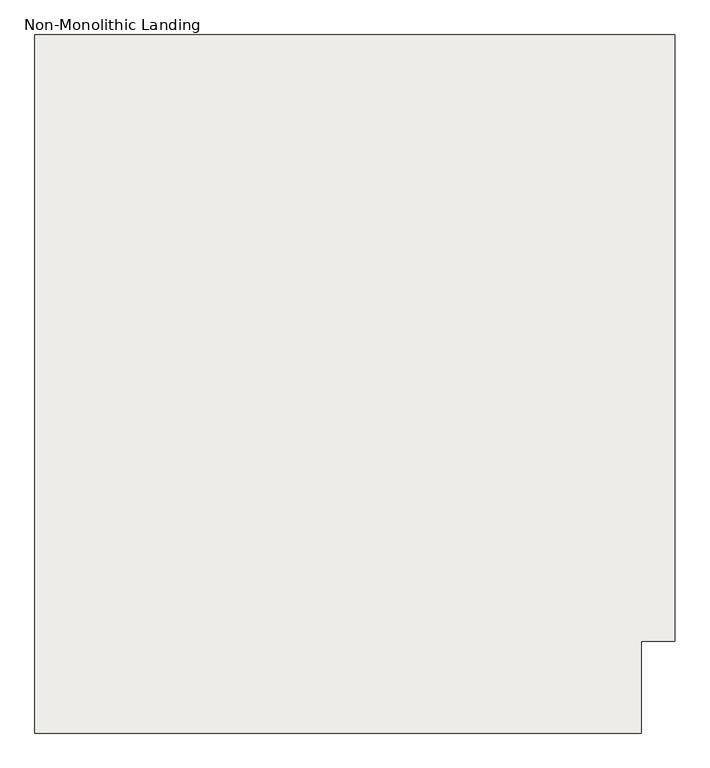
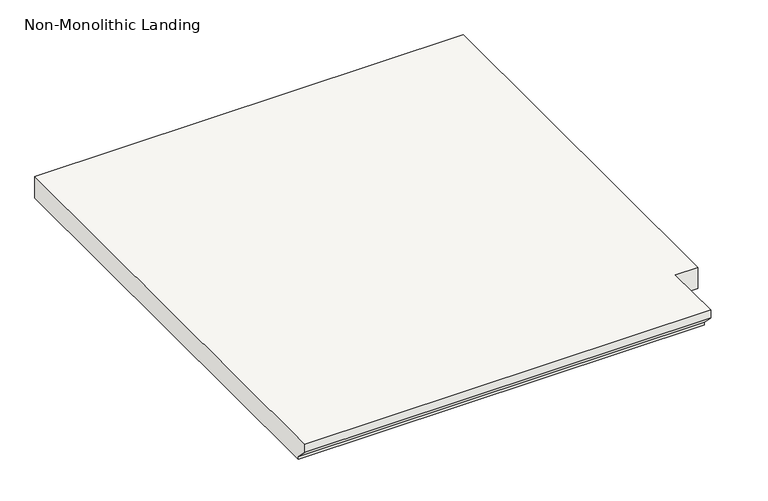
"""IFC4 building model written with IfcOpenShell, lengths in millimetres: slab geometry, Non-Monolithic Landing."""

from ifc_helpers import new_model, si_unit, origin, place, context, project, spatial, faceted_brep, source, transform, mapped, element, save


def non_monolithic_landing_d7f15ac0(model_context):
    return source(origin(), model_context, "Body", "Brep", [
        faceted_brep([(-14022.18283, 7638.1500793, 3875.6166667), (-14022.18283, 7638.1500793, 3894.6666667), (-14936.58283, 7638.1500793, 3894.6666667), (-14936.58283, 7638.1500793, 3875.6166667), (-14022.18283, 7663.5500793, 3850.2166667), (-14936.58283, 7663.5500793, 3850.2166667), (-14022.18283, 7777.0620171, 3894.6666667), (-13971.38283, 7777.0620171, 3894.6666667), (-13971.38283, 8691.4620171, 3894.6666667), (-14936.58283, 8691.4620171, 3894.6666667), (-14022.18283, 7663.5500793, 3843.8666667), (-14936.58283, 7663.5500793, 3843.8666667), (-14936.58283, 8691.4620171, 3843.8666667), (-13971.38283, 8691.4620171, 3843.8666667), (-13971.38283, 7777.0620171, 3843.8666667), (-14022.18283, 7777.0620171, 3843.8666667)], [[[0, 1, 2, 3]], [[4, 0, 3, 5]], [[6, 7, 8, 9, 2, 1]], [[10, 11, 12, 13, 14, 15]], [[11, 10, 4, 5]], [[6, 1, 0, 4, 10, 15]], [[7, 6, 15, 14]], [[9, 8, 13, 12]], [[2, 9, 12, 11, 5, 3]], [[8, 7, 14, 13]]]),
    ])


if __name__ == "__main__":
    model = new_model("IFC4")
    model_context = context("Model", 3, world=origin())
    ifc_project = project(units=[si_unit("LENGTHUNIT", "METRE", prefix="MILLI")], contexts=[model_context])
    site = spatial("IfcSite", under=ifc_project)
    building = spatial("IfcBuilding", under=site)
    placement = place(None, origin())
    non_monolithic_landing_shape = non_monolithic_landing_d7f15ac0(model_context)
    element("IfcSlab", 1, ObjectType="Non-Monolithic Landing", at=placement, inside=building, context=model_context, shape_type="MappedRepresentation", body=[
        mapped(non_monolithic_landing_shape, transform((0.0, 0.0, 0.0), x_axis=(1.0, 0.0, 0.0), y_axis=(0.0, 1.0, 0.0), z_axis=(0.0, 0.0, 1.0))),
    ])
    save(model, "model.ifc")
